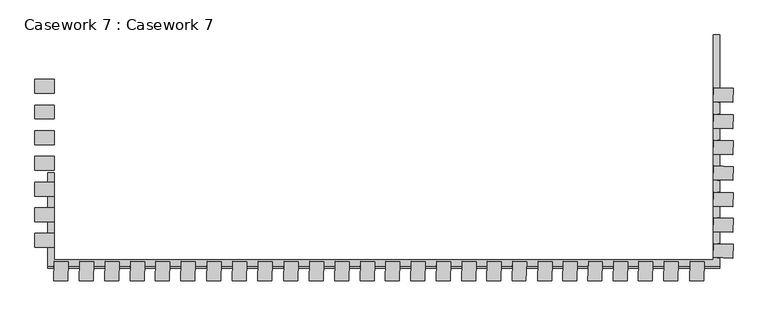
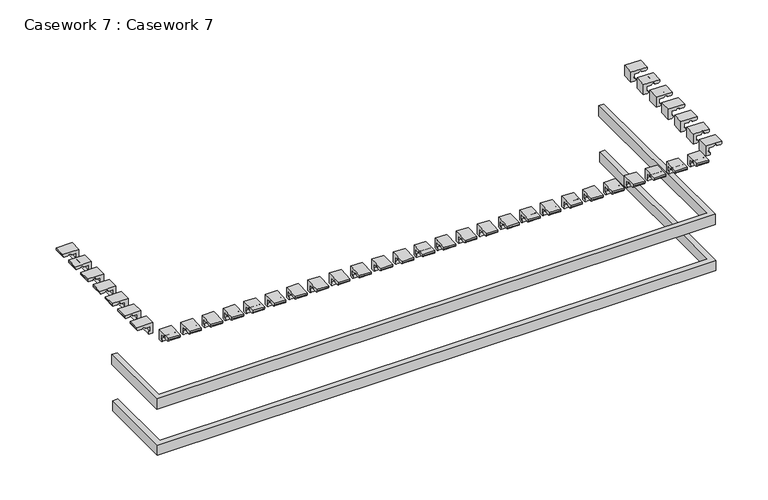
"""IFC4 building model written with IfcOpenShell, lengths in millimetres: furniture geometry, Casework 7 : Casework 7."""

from ifc_helpers import new_model, si_unit, point, frame, frame_2d, origin, place, context, project, spatial, polyline, circle_curve, trimmed, segment, composite_curve, outline, extrude, source, transform, mapped, element, save


def casework_7_casework_7_7bbf8f76(model_context):
    return source(origin(), model_context, "Body", "SweptSolid", [
        extrude(outline(composite_curve([segment(polyline([(0.0, 0.0), (15.0, 0.0)]), True, "CONTINUOUS"), segment(trimmed(circle_curve(frame_2d((15.0, -15.0)), 15.0), [point((15.0, 0.0))], [point((30.0, -15.0))], False, "CARTESIAN"), True, "CONTINUOUS"), segment(polyline([(30.0, -15.0), (30.0, -47.4999999)]), True, "CONTINUOUS"), segment(trimmed(circle_curve(frame_2d((30.0, -62.4999999)), 15.0), [point((30.0, -47.4999999))], [point((30.0, -77.5))], True, "CARTESIAN"), True, "CONTINUOUS"), segment(polyline([(30.0, -77.5), (30.0, -120.0), (70.0, -120.0)]), True, "CONTINUOUS"), segment(trimmed(circle_curve(frame_2d((85.0, -120.0)), 15.0), [point((70.0, -120.0))], [point((100.0, -120.0))], False, "CARTESIAN"), True, "CONTINUOUS"), segment(polyline([(100.0, -120.0), (100.0, -150.0), (0.0, -150.0), (0.0, 0.0)]), True, "CONTINUOUS")], self_intersect=False)), frame((3179.6256879, -13036.8692678, 4349.8564029), z_axis=(-0.9996210812387005, 0.02752624099239521, 0.0), x_axis=(0.0, 0.0, -1.0)), (0.0, 0.0, 1.0), 108.7993469),
        extrude(outline(composite_curve([segment(polyline([(0.0, 0.0), (15.0, 0.0)]), True, "CONTINUOUS"), segment(trimmed(circle_curve(frame_2d((15.0, -15.0)), 15.0), [point((15.0, 0.0))], [point((30.0, -15.0))], False, "CARTESIAN"), True, "CONTINUOUS"), segment(polyline([(30.0, -15.0), (30.0, -47.4999999)]), True, "CONTINUOUS"), segment(trimmed(circle_curve(frame_2d((30.0, -62.4999999)), 15.0), [point((30.0, -47.4999999))], [point((30.0, -77.5))], True, "CARTESIAN"), True, "CONTINUOUS"), segment(polyline([(30.0, -77.5), (30.0, -120.0), (70.0, -120.0)]), True, "CONTINUOUS"), segment(trimmed(circle_curve(frame_2d((85.0, -120.0)), 15.0), [point((70.0, -120.0))], [point((100.0, -120.0))], False, "CARTESIAN"), True, "CONTINUOUS"), segment(polyline([(100.0, -120.0), (100.0, -150.0), (0.0, -150.0), (0.0, 0.0)]), True, "CONTINUOUS")], self_intersect=False)), frame((2979.6256879, -13036.8692678, 4349.8564029), z_axis=(-0.9996210812387005, 0.02752624099239521, 0.0), x_axis=(0.0, 0.0, -1.0)), (0.0, 0.0, 1.0), 108.7993469),
        extrude(outline(composite_curve([segment(polyline([(0.0, 0.0), (15.0, 0.0)]), True, "CONTINUOUS"), segment(trimmed(circle_curve(frame_2d((15.0, -15.0)), 15.0), [point((15.0, 0.0))], [point((30.0, -15.0))], False, "CARTESIAN"), True, "CONTINUOUS"), segment(polyline([(30.0, -15.0), (30.0, -47.4999999)]), True, "CONTINUOUS"), segment(trimmed(circle_curve(frame_2d((30.0, -62.4999999)), 15.0), [point((30.0, -47.4999999))], [point((30.0, -77.5))], True, "CARTESIAN"), True, "CONTINUOUS"), segment(polyline([(30.0, -77.5), (30.0, -120.0), (70.0, -120.0)]), True, "CONTINUOUS"), segment(trimmed(circle_curve(frame_2d((85.0, -120.0)), 15.0), [point((70.0, -120.0))], [point((100.0, -120.0))], False, "CARTESIAN"), True, "CONTINUOUS"), segment(polyline([(100.0, -120.0), (100.0, -150.0), (0.0, -150.0), (0.0, 0.0)]), True, "CONTINUOUS")], self_intersect=False)), frame((2779.6256879, -13036.8692678, 4349.8564029), z_axis=(-0.9996210812387005, 0.02752624099239521, 0.0), x_axis=(0.0, 0.0, -1.0)), (0.0, 0.0, 1.0), 108.7993469),
        extrude(outline(composite_curve([segment(polyline([(0.0, 0.0), (15.0, 0.0)]), True, "CONTINUOUS"), segment(trimmed(circle_curve(frame_2d((15.0, -15.0)), 15.0), [point((15.0, 0.0))], [point((30.0, -15.0))], False, "CARTESIAN"), True, "CONTINUOUS"), segment(polyline([(30.0, -15.0), (30.0, -47.4999999)]), True, "CONTINUOUS"), segment(trimmed(circle_curve(frame_2d((30.0, -62.4999999)), 15.0), [point((30.0, -47.4999999))], [point((30.0, -77.5))], True, "CARTESIAN"), True, "CONTINUOUS"), segment(polyline([(30.0, -77.5), (30.0, -120.0), (70.0, -120.0)]), True, "CONTINUOUS"), segment(trimmed(circle_curve(frame_2d((85.0, -120.0)), 15.0), [point((70.0, -120.0))], [point((100.0, -120.0))], False, "CARTESIAN"), True, "CONTINUOUS"), segment(polyline([(100.0, -120.0), (100.0, -150.0), (0.0, -150.0), (0.0, 0.0)]), True, "CONTINUOUS")], self_intersect=False)), frame((2583.754624, -13036.8692678, 4349.8564029), z_axis=(-0.9996210812387005, 0.02752624099239521, 0.0), x_axis=(0.0, 0.0, -1.0)), (0.0, 0.0, 1.0), 108.7993469),
        extrude(outline(composite_curve([segment(polyline([(0.0, 0.0), (15.0, 0.0)]), True, "CONTINUOUS"), segment(trimmed(circle_curve(frame_2d((15.0, -15.0)), 15.0), [point((15.0, 0.0))], [point((30.0, -15.0))], False, "CARTESIAN"), True, "CONTINUOUS"), segment(polyline([(30.0, -15.0), (30.0, -47.4999999)]), True, "CONTINUOUS"), segment(trimmed(circle_curve(frame_2d((30.0, -62.4999999)), 15.0), [point((30.0, -47.4999999))], [point((30.0, -77.5))], True, "CARTESIAN"), True, "CONTINUOUS"), segment(polyline([(30.0, -77.5), (30.0, -120.0), (70.0, -120.0)]), True, "CONTINUOUS"), segment(trimmed(circle_curve(frame_2d((85.0, -120.0)), 15.0), [point((70.0, -120.0))], [point((100.0, -120.0))], False, "CARTESIAN"), True, "CONTINUOUS"), segment(polyline([(100.0, -120.0), (100.0, -150.0), (0.0, -150.0), (0.0, 0.0)]), True, "CONTINUOUS")], self_intersect=False)), frame((2387.8835602, -13036.8692678, 4349.8564029), z_axis=(-0.9996210812387005, 0.02752624099239521, 0.0), x_axis=(0.0, 0.0, -1.0)), (0.0, 0.0, 1.0), 108.7993469),
        extrude(outline(composite_curve([segment(polyline([(0.0, 0.0), (15.0, 0.0)]), True, "CONTINUOUS"), segment(trimmed(circle_curve(frame_2d((15.0, -15.0)), 15.0), [point((15.0, 0.0))], [point((30.0, -15.0))], False, "CARTESIAN"), True, "CONTINUOUS"), segment(polyline([(30.0, -15.0), (30.0, -47.4999999)]), True, "CONTINUOUS"), segment(trimmed(circle_curve(frame_2d((30.0, -62.4999999)), 15.0), [point((30.0, -47.4999999))], [point((30.0, -77.5))], True, "CARTESIAN"), True, "CONTINUOUS"), segment(polyline([(30.0, -77.5), (30.0, -120.0), (70.0, -120.0)]), True, "CONTINUOUS"), segment(trimmed(circle_curve(frame_2d((85.0, -120.0)), 15.0), [point((70.0, -120.0))], [point((100.0, -120.0))], False, "CARTESIAN"), True, "CONTINUOUS"), segment(polyline([(100.0, -120.0), (100.0, -150.0), (0.0, -150.0), (0.0, 0.0)]), True, "CONTINUOUS")], self_intersect=False)), frame((2192.0124963, -13036.8692678, 4349.8564029), z_axis=(-0.9996210812387005, 0.02752624099239521, 0.0), x_axis=(0.0, 0.0, -1.0)), (0.0, 0.0, 1.0), 108.7993469),
        extrude(outline(composite_curve([segment(polyline([(0.0, 0.0), (15.0, 0.0)]), True, "CONTINUOUS"), segment(trimmed(circle_curve(frame_2d((15.0, -15.0)), 15.0), [point((15.0, 0.0))], [point((30.0, -15.0))], False, "CARTESIAN"), True, "CONTINUOUS"), segment(polyline([(30.0, -15.0), (30.0, -47.4999999)]), True, "CONTINUOUS"), segment(trimmed(circle_curve(frame_2d((30.0, -62.4999999)), 15.0), [point((30.0, -47.4999999))], [point((30.0, -77.5))], True, "CARTESIAN"), True, "CONTINUOUS"), segment(polyline([(30.0, -77.5), (30.0, -120.0), (70.0, -120.0)]), True, "CONTINUOUS"), segment(trimmed(circle_curve(frame_2d((85.0, -120.0)), 15.0), [point((70.0, -120.0))], [point((100.0, -120.0))], False, "CARTESIAN"), True, "CONTINUOUS"), segment(polyline([(100.0, -120.0), (100.0, -150.0), (0.0, -150.0), (0.0, 0.0)]), True, "CONTINUOUS")], self_intersect=False)), frame((1996.1414325, -13036.8692678, 4349.8564029), z_axis=(-0.9996210812387005, 0.02752624099239521, 0.0), x_axis=(0.0, 0.0, -1.0)), (0.0, 0.0, 1.0), 108.7993469),
        extrude(outline(composite_curve([segment(polyline([(0.0, 0.0), (15.0, 0.0)]), True, "CONTINUOUS"), segment(trimmed(circle_curve(frame_2d((15.0, -15.0)), 15.0), [point((15.0, 0.0))], [point((30.0, -15.0))], False, "CARTESIAN"), True, "CONTINUOUS"), segment(polyline([(30.0, -15.0), (30.0, -47.4999999)]), True, "CONTINUOUS"), segment(trimmed(circle_curve(frame_2d((30.0, -62.4999999)), 15.0), [point((30.0, -47.4999999))], [point((30.0, -77.5))], True, "CARTESIAN"), True, "CONTINUOUS"), segment(polyline([(30.0, -77.5), (30.0, -120.0), (70.0, -120.0)]), True, "CONTINUOUS"), segment(trimmed(circle_curve(frame_2d((85.0, -120.0)), 15.0), [point((70.0, -120.0))], [point((100.0, -120.0))], False, "CARTESIAN"), True, "CONTINUOUS"), segment(polyline([(100.0, -120.0), (100.0, -150.0), (0.0, -150.0), (0.0, 0.0)]), True, "CONTINUOUS")], self_intersect=False)), frame((1796.1414325, -13036.8692678, 4349.8564029), z_axis=(-0.9996210812387005, 0.02752624099239521, 0.0), x_axis=(0.0, 0.0, -1.0)), (0.0, 0.0, 1.0), 108.7993469),
        extrude(outline(composite_curve([segment(polyline([(0.0, 0.0), (15.0, 0.0)]), True, "CONTINUOUS"), segment(trimmed(circle_curve(frame_2d((15.0, -15.0)), 15.0), [point((15.0, 0.0))], [point((30.0, -15.0))], False, "CARTESIAN"), True, "CONTINUOUS"), segment(polyline([(30.0, -15.0), (30.0, -47.4999999)]), True, "CONTINUOUS"), segment(trimmed(circle_curve(frame_2d((30.0, -62.4999999)), 15.0), [point((30.0, -47.4999999))], [point((30.0, -77.5))], True, "CARTESIAN"), True, "CONTINUOUS"), segment(polyline([(30.0, -77.5), (30.0, -120.0), (70.0, -120.0)]), True, "CONTINUOUS"), segment(trimmed(circle_curve(frame_2d((85.0, -120.0)), 15.0), [point((70.0, -120.0))], [point((100.0, -120.0))], False, "CARTESIAN"), True, "CONTINUOUS"), segment(polyline([(100.0, -120.0), (100.0, -150.0), (0.0, -150.0), (0.0, 0.0)]), True, "CONTINUOUS")], self_intersect=False)), frame((1600.2703686, -13036.8692678, 4349.8564029), z_axis=(-0.9996210812387005, 0.02752624099239521, 0.0), x_axis=(0.0, 0.0, -1.0)), (0.0, 0.0, 1.0), 108.7993469),
        extrude(outline(composite_curve([segment(polyline([(0.0, 0.0), (15.0, 0.0)]), True, "CONTINUOUS"), segment(trimmed(circle_curve(frame_2d((15.0, -15.0)), 15.0), [point((15.0, 0.0))], [point((30.0, -15.0))], False, "CARTESIAN"), True, "CONTINUOUS"), segment(polyline([(30.0, -15.0), (30.0, -47.4999999)]), True, "CONTINUOUS"), segment(trimmed(circle_curve(frame_2d((30.0, -62.4999999)), 15.0), [point((30.0, -47.4999999))], [point((30.0, -77.5))], True, "CARTESIAN"), True, "CONTINUOUS"), segment(polyline([(30.0, -77.5), (30.0, -120.0), (70.0, -120.0)]), True, "CONTINUOUS"), segment(trimmed(circle_curve(frame_2d((85.0, -120.0)), 15.0), [point((70.0, -120.0))], [point((100.0, -120.0))], False, "CARTESIAN"), True, "CONTINUOUS"), segment(polyline([(100.0, -120.0), (100.0, -150.0), (0.0, -150.0), (0.0, 0.0)]), True, "CONTINUOUS")], self_intersect=False)), frame((1404.3993048, -13036.8692678, 4349.8564029), z_axis=(-0.9996210812387005, 0.02752624099239521, 0.0), x_axis=(0.0, 0.0, -1.0)), (0.0, 0.0, 1.0), 108.7993469),
        extrude(outline(composite_curve([segment(polyline([(0.0, 0.0), (15.0, 0.0)]), True, "CONTINUOUS"), segment(trimmed(circle_curve(frame_2d((15.0, -15.0)), 15.0), [point((15.0, 0.0))], [point((30.0, -15.0))], False, "CARTESIAN"), True, "CONTINUOUS"), segment(polyline([(30.0, -15.0), (30.0, -47.4999999)]), True, "CONTINUOUS"), segment(trimmed(circle_curve(frame_2d((30.0, -62.4999999)), 15.0), [point((30.0, -47.4999999))], [point((30.0, -77.5))], True, "CARTESIAN"), True, "CONTINUOUS"), segment(polyline([(30.0, -77.5), (30.0, -120.0), (70.0, -120.0)]), True, "CONTINUOUS"), segment(trimmed(circle_curve(frame_2d((85.0, -120.0)), 15.0), [point((70.0, -120.0))], [point((100.0, -120.0))], False, "CARTESIAN"), True, "CONTINUOUS"), segment(polyline([(100.0, -120.0), (100.0, -150.0), (0.0, -150.0), (0.0, 0.0)]), True, "CONTINUOUS")], self_intersect=False)), frame((1204.3993048, -13036.8692678, 4349.8564029), z_axis=(-0.9996210812387005, 0.02752624099239521, 0.0), x_axis=(0.0, 0.0, -1.0)), (0.0, 0.0, 1.0), 108.7993469),
        extrude(outline(composite_curve([segment(polyline([(0.0, 0.0), (15.0, 0.0)]), True, "CONTINUOUS"), segment(trimmed(circle_curve(frame_2d((15.0, -15.0)), 15.0), [point((15.0, 0.0))], [point((30.0, -15.0))], False, "CARTESIAN"), True, "CONTINUOUS"), segment(polyline([(30.0, -15.0), (30.0, -47.4999999)]), True, "CONTINUOUS"), segment(trimmed(circle_curve(frame_2d((30.0, -62.4999999)), 15.0), [point((30.0, -47.4999999))], [point((30.0, -77.5))], True, "CARTESIAN"), True, "CONTINUOUS"), segment(polyline([(30.0, -77.5), (30.0, -120.0), (70.0, -120.0)]), True, "CONTINUOUS"), segment(trimmed(circle_curve(frame_2d((85.0, -120.0)), 15.0), [point((70.0, -120.0))], [point((100.0, -120.0))], False, "CARTESIAN"), True, "CONTINUOUS"), segment(polyline([(100.0, -120.0), (100.0, -150.0), (0.0, -150.0), (0.0, 0.0)]), True, "CONTINUOUS")], self_intersect=False)), frame((1008.5282409, -13036.8692678, 4349.8564029), z_axis=(-0.9996210812387005, 0.02752624099239521, 0.0), x_axis=(0.0, 0.0, -1.0)), (0.0, 0.0, 1.0), 108.7993469),
        extrude(outline(composite_curve([segment(polyline([(0.0, 0.0), (15.0, 0.0)]), True, "CONTINUOUS"), segment(trimmed(circle_curve(frame_2d((15.0, -15.0)), 15.0), [point((15.0, 0.0))], [point((30.0, -15.0))], False, "CARTESIAN"), True, "CONTINUOUS"), segment(polyline([(30.0, -15.0), (30.0, -47.4999999)]), True, "CONTINUOUS"), segment(trimmed(circle_curve(frame_2d((30.0, -62.4999999)), 15.0), [point((30.0, -47.4999999))], [point((30.0, -77.5))], True, "CARTESIAN"), True, "CONTINUOUS"), segment(polyline([(30.0, -77.5), (30.0, -120.0), (70.0, -120.0)]), True, "CONTINUOUS"), segment(trimmed(circle_curve(frame_2d((85.0, -120.0)), 15.0), [point((70.0, -120.0))], [point((100.0, -120.0))], False, "CARTESIAN"), True, "CONTINUOUS"), segment(polyline([(100.0, -120.0), (100.0, -150.0), (0.0, -150.0), (0.0, 0.0)]), True, "CONTINUOUS")], self_intersect=False)), frame((808.5282409, -13036.8692678, 4349.8564029), z_axis=(-0.9996210812387005, 0.02752624099239521, 0.0), x_axis=(0.0, 0.0, -1.0)), (0.0, 0.0, 1.0), 108.7993469),
        extrude(outline(composite_curve([segment(polyline([(0.0, 0.0), (15.0, 0.0)]), True, "CONTINUOUS"), segment(trimmed(circle_curve(frame_2d((15.0, -15.0)), 15.0), [point((15.0, 0.0))], [point((30.0, -15.0))], False, "CARTESIAN"), True, "CONTINUOUS"), segment(polyline([(30.0, -15.0), (30.0, -47.4999999)]), True, "CONTINUOUS"), segment(trimmed(circle_curve(frame_2d((30.0, -62.4999999)), 15.0), [point((30.0, -47.4999999))], [point((30.0, -77.5))], True, "CARTESIAN"), True, "CONTINUOUS"), segment(polyline([(30.0, -77.5), (30.0, -120.0), (70.0, -120.0)]), True, "CONTINUOUS"), segment(trimmed(circle_curve(frame_2d((85.0, -120.0)), 15.0), [point((70.0, -120.0))], [point((100.0, -120.0))], False, "CARTESIAN"), True, "CONTINUOUS"), segment(polyline([(100.0, -120.0), (100.0, -150.0), (0.0, -150.0), (0.0, 0.0)]), True, "CONTINUOUS")], self_intersect=False)), frame((612.6571771, -13036.8692678, 4349.8564029), z_axis=(-0.9996210812387005, 0.02752624099239521, 0.0), x_axis=(0.0, 0.0, -1.0)), (0.0, 0.0, 1.0), 108.7993469),
        extrude(outline(composite_curve([segment(polyline([(0.0, 0.0), (15.0, 0.0)]), True, "CONTINUOUS"), segment(trimmed(circle_curve(frame_2d((15.0, -15.0)), 15.0), [point((15.0, 0.0))], [point((30.0, -15.0))], False, "CARTESIAN"), True, "CONTINUOUS"), segment(polyline([(30.0, -15.0), (30.0, -47.4999999)]), True, "CONTINUOUS"), segment(trimmed(circle_curve(frame_2d((30.0, -62.4999999)), 15.0), [point((30.0, -47.4999999))], [point((30.0, -77.5))], True, "CARTESIAN"), True, "CONTINUOUS"), segment(polyline([(30.0, -77.5), (30.0, -120.0), (70.0, -120.0)]), True, "CONTINUOUS"), segment(trimmed(circle_curve(frame_2d((85.0, -120.0)), 15.0), [point((70.0, -120.0))], [point((100.0, -120.0))], False, "CARTESIAN"), True, "CONTINUOUS"), segment(polyline([(100.0, -120.0), (100.0, -150.0), (0.0, -150.0), (0.0, 0.0)]), True, "CONTINUOUS")], self_intersect=False)), frame((416.7861132, -13036.8692678, 4349.8564029), z_axis=(-0.9996210812387005, 0.02752624099239521, 0.0), x_axis=(0.0, 0.0, -1.0)), (0.0, 0.0, 1.0), 108.7993469),
        extrude(outline(composite_curve([segment(polyline([(0.0, 0.0), (15.0, 0.0)]), True, "CONTINUOUS"), segment(trimmed(circle_curve(frame_2d((15.0, -15.0)), 15.0), [point((15.0, 0.0))], [point((30.0, -15.0))], False, "CARTESIAN"), True, "CONTINUOUS"), segment(polyline([(30.0, -15.0), (30.0, -47.4999999)]), True, "CONTINUOUS"), segment(trimmed(circle_curve(frame_2d((30.0, -62.4999999)), 15.0), [point((30.0, -47.4999999))], [point((30.0, -77.5))], True, "CARTESIAN"), True, "CONTINUOUS"), segment(polyline([(30.0, -77.5), (30.0, -120.0), (70.0, -120.0)]), True, "CONTINUOUS"), segment(trimmed(circle_curve(frame_2d((85.0, -120.0)), 15.0), [point((70.0, -120.0))], [point((100.0, -120.0))], False, "CARTESIAN"), True, "CONTINUOUS"), segment(polyline([(100.0, -120.0), (100.0, -150.0), (0.0, -150.0), (0.0, 0.0)]), True, "CONTINUOUS")], self_intersect=False)), frame((216.7861132, -13036.8692678, 4349.8564029), z_axis=(-0.9996210812387005, 0.02752624099239521, 0.0), x_axis=(0.0, 0.0, -1.0)), (0.0, 0.0, 1.0), 108.7993469),
        extrude(outline(composite_curve([segment(polyline([(0.0, 0.0), (15.0, 0.0)]), True, "CONTINUOUS"), segment(trimmed(circle_curve(frame_2d((15.0, -15.0)), 15.0), [point((15.0, 0.0))], [point((30.0, -15.0))], False, "CARTESIAN"), True, "CONTINUOUS"), segment(polyline([(30.0, -15.0), (30.0, -47.4999999)]), True, "CONTINUOUS"), segment(trimmed(circle_curve(frame_2d((30.0, -62.4999999)), 15.0), [point((30.0, -47.4999999))], [point((30.0, -77.5))], True, "CARTESIAN"), True, "CONTINUOUS"), segment(polyline([(30.0, -77.5), (30.0, -120.0), (70.0, -120.0)]), True, "CONTINUOUS"), segment(trimmed(circle_curve(frame_2d((85.0, -120.0)), 15.0), [point((70.0, -120.0))], [point((100.0, -120.0))], False, "CARTESIAN"), True, "CONTINUOUS"), segment(polyline([(100.0, -120.0), (100.0, -150.0), (0.0, -150.0), (0.0, 0.0)]), True, "CONTINUOUS")], self_intersect=False)), frame((16.7861132, -13036.8692678, 4349.8564029), z_axis=(-0.9996210812387005, 0.02752624099239521, 0.0), x_axis=(0.0, 0.0, -1.0)), (0.0, 0.0, 1.0), 108.7993469),
        extrude(outline(composite_curve([segment(polyline([(0.0, 0.0), (15.0, 0.0)]), True, "CONTINUOUS"), segment(trimmed(circle_curve(frame_2d((15.0, -15.0)), 15.0), [point((15.0, 0.0))], [point((30.0, -15.0))], False, "CARTESIAN"), True, "CONTINUOUS"), segment(polyline([(30.0, -15.0), (30.0, -47.4999999)]), True, "CONTINUOUS"), segment(trimmed(circle_curve(frame_2d((30.0, -62.4999999)), 15.0), [point((30.0, -47.4999999))], [point((30.0, -77.5))], True, "CARTESIAN"), True, "CONTINUOUS"), segment(polyline([(30.0, -77.5), (30.0, -120.0), (70.0, -120.0)]), True, "CONTINUOUS"), segment(trimmed(circle_curve(frame_2d((85.0, -120.0)), 15.0), [point((70.0, -120.0))], [point((100.0, -120.0))], False, "CARTESIAN"), True, "CONTINUOUS"), segment(polyline([(100.0, -120.0), (100.0, -150.0), (0.0, -150.0), (0.0, 0.0)]), True, "CONTINUOUS")], self_intersect=False)), frame((-183.2138868, -13036.8692678, 4349.8564029), z_axis=(-0.9996210812387005, 0.02752624099239521, 0.0), x_axis=(0.0, 0.0, -1.0)), (0.0, 0.0, 1.0), 108.7993469),
        extrude(outline(composite_curve([segment(polyline([(0.0, 0.0), (15.0, 0.0)]), True, "CONTINUOUS"), segment(trimmed(circle_curve(frame_2d((15.0, -15.0)), 15.0), [point((15.0, 0.0))], [point((30.0, -15.0))], False, "CARTESIAN"), True, "CONTINUOUS"), segment(polyline([(30.0, -15.0), (30.0, -47.4999999)]), True, "CONTINUOUS"), segment(trimmed(circle_curve(frame_2d((30.0, -62.4999999)), 15.0), [point((30.0, -47.4999999))], [point((30.0, -77.5))], True, "CARTESIAN"), True, "CONTINUOUS"), segment(polyline([(30.0, -77.5), (30.0, -120.0), (70.0, -120.0)]), True, "CONTINUOUS"), segment(trimmed(circle_curve(frame_2d((85.0, -120.0)), 15.0), [point((70.0, -120.0))], [point((100.0, -120.0))], False, "CARTESIAN"), True, "CONTINUOUS"), segment(polyline([(100.0, -120.0), (100.0, -150.0), (0.0, -150.0), (0.0, 0.0)]), True, "CONTINUOUS")], self_intersect=False)), frame((-383.2138868, -13036.8692678, 4349.8564029), z_axis=(-0.9996210812387005, 0.02752624099239521, 0.0), x_axis=(0.0, 0.0, -1.0)), (0.0, 0.0, 1.0), 108.7993469),
        extrude(outline(composite_curve([segment(polyline([(0.0, 0.0), (15.0, 0.0)]), True, "CONTINUOUS"), segment(trimmed(circle_curve(frame_2d((15.0, -15.0)), 15.0), [point((15.0, 0.0))], [point((30.0, -15.0))], False, "CARTESIAN"), True, "CONTINUOUS"), segment(polyline([(30.0, -15.0), (30.0, -47.4999999)]), True, "CONTINUOUS"), segment(trimmed(circle_curve(frame_2d((30.0, -62.4999999)), 15.0), [point((30.0, -47.4999999))], [point((30.0, -77.5))], True, "CARTESIAN"), True, "CONTINUOUS"), segment(polyline([(30.0, -77.5), (30.0, -120.0), (70.0, -120.0)]), True, "CONTINUOUS"), segment(trimmed(circle_curve(frame_2d((85.0, -120.0)), 15.0), [point((70.0, -120.0))], [point((100.0, -120.0))], False, "CARTESIAN"), True, "CONTINUOUS"), segment(polyline([(100.0, -120.0), (100.0, -150.0), (0.0, -150.0), (0.0, 0.0)]), True, "CONTINUOUS")], self_intersect=False)), frame((-583.2138868, -13036.8692678, 4349.8564029), z_axis=(-0.9996210812387005, 0.02752624099239521, 0.0), x_axis=(0.0, 0.0, -1.0)), (0.0, 0.0, 1.0), 108.7993469),
        extrude(outline(composite_curve([segment(polyline([(0.0, 0.0), (15.0, 0.0)]), True, "CONTINUOUS"), segment(trimmed(circle_curve(frame_2d((15.0, -15.0)), 15.0), [point((15.0, 0.0))], [point((30.0, -15.0))], False, "CARTESIAN"), True, "CONTINUOUS"), segment(polyline([(30.0, -15.0), (30.0, -47.4999999)]), True, "CONTINUOUS"), segment(trimmed(circle_curve(frame_2d((30.0, -62.4999999)), 15.0), [point((30.0, -47.4999999))], [point((30.0, -77.5))], True, "CARTESIAN"), True, "CONTINUOUS"), segment(polyline([(30.0, -77.5), (30.0, -120.0), (70.0, -120.0)]), True, "CONTINUOUS"), segment(trimmed(circle_curve(frame_2d((85.0, -120.0)), 15.0), [point((70.0, -120.0))], [point((100.0, -120.0))], False, "CARTESIAN"), True, "CONTINUOUS"), segment(polyline([(100.0, -120.0), (100.0, -150.0), (0.0, -150.0), (0.0, 0.0)]), True, "CONTINUOUS")], self_intersect=False)), frame((-783.2138868, -13036.8692678, 4349.8564029), z_axis=(-0.9996210812387005, 0.02752624099239521, 0.0), x_axis=(0.0, 0.0, -1.0)), (0.0, 0.0, 1.0), 108.7993469),
        extrude(outline(composite_curve([segment(polyline([(0.0, 0.0), (15.0, 0.0)]), True, "CONTINUOUS"), segment(trimmed(circle_curve(frame_2d((15.0, -15.0)), 15.0), [point((15.0, 0.0))], [point((30.0, -15.0))], False, "CARTESIAN"), True, "CONTINUOUS"), segment(polyline([(30.0, -15.0), (30.0, -47.4999999)]), True, "CONTINUOUS"), segment(trimmed(circle_curve(frame_2d((30.0, -62.4999999)), 15.0), [point((30.0, -47.4999999))], [point((30.0, -77.5))], True, "CARTESIAN"), True, "CONTINUOUS"), segment(polyline([(30.0, -77.5), (30.0, -120.0), (70.0, -120.0)]), True, "CONTINUOUS"), segment(trimmed(circle_curve(frame_2d((85.0, -120.0)), 15.0), [point((70.0, -120.0))], [point((100.0, -120.0))], False, "CARTESIAN"), True, "CONTINUOUS"), segment(polyline([(100.0, -120.0), (100.0, -150.0), (0.0, -150.0), (0.0, 0.0)]), True, "CONTINUOUS")], self_intersect=False)), frame((-983.2138868, -13036.8692678, 4349.8564029), z_axis=(-0.9996210812387005, 0.02752624099239521, 0.0), x_axis=(0.0, 0.0, -1.0)), (0.0, 0.0, 1.0), 108.7993469),
        extrude(outline(composite_curve([segment(polyline([(0.0, 0.0), (15.0, 0.0)]), True, "CONTINUOUS"), segment(trimmed(circle_curve(frame_2d((15.0, -15.0)), 15.0), [point((15.0, 0.0))], [point((30.0, -15.0))], False, "CARTESIAN"), True, "CONTINUOUS"), segment(polyline([(30.0, -15.0), (30.0, -47.4999999)]), True, "CONTINUOUS"), segment(trimmed(circle_curve(frame_2d((30.0, -62.4999999)), 15.0), [point((30.0, -47.4999999))], [point((30.0, -77.5))], True, "CARTESIAN"), True, "CONTINUOUS"), segment(polyline([(30.0, -77.5), (30.0, -120.0), (70.0, -120.0)]), True, "CONTINUOUS"), segment(trimmed(circle_curve(frame_2d((85.0, -120.0)), 15.0), [point((70.0, -120.0))], [point((100.0, -120.0))], False, "CARTESIAN"), True, "CONTINUOUS"), segment(polyline([(100.0, -120.0), (100.0, -150.0), (0.0, -150.0), (0.0, 0.0)]), True, "CONTINUOUS")], self_intersect=False)), frame((-1179.0849506, -13036.8692678, 4349.8564029), z_axis=(-0.9996210812387005, 0.02752624099239521, 0.0), x_axis=(0.0, 0.0, -1.0)), (0.0, 0.0, 1.0), 108.7993469),
        extrude(outline(composite_curve([segment(polyline([(0.0, 0.0), (15.0, 0.0)]), True, "CONTINUOUS"), segment(trimmed(circle_curve(frame_2d((15.0, -15.0)), 15.0), [point((15.0, 0.0))], [point((30.0, -15.0))], False, "CARTESIAN"), True, "CONTINUOUS"), segment(polyline([(30.0, -15.0), (30.0, -47.4999999)]), True, "CONTINUOUS"), segment(trimmed(circle_curve(frame_2d((30.0, -62.4999999)), 15.0), [point((30.0, -47.4999999))], [point((30.0, -77.5))], True, "CARTESIAN"), True, "CONTINUOUS"), segment(polyline([(30.0, -77.5), (30.0, -120.0), (70.0, -120.0)]), True, "CONTINUOUS"), segment(trimmed(circle_curve(frame_2d((85.0, -120.0)), 15.0), [point((70.0, -120.0))], [point((100.0, -120.0))], False, "CARTESIAN"), True, "CONTINUOUS"), segment(polyline([(100.0, -120.0), (100.0, -150.0), (0.0, -150.0), (0.0, 0.0)]), True, "CONTINUOUS")], self_intersect=False)), frame((-1374.9560145, -13036.8692678, 4349.8564029), z_axis=(-0.9996210812387005, 0.02752624099239521, 0.0), x_axis=(0.0, 0.0, -1.0)), (0.0, 0.0, 1.0), 108.7993469),
        extrude(outline(composite_curve([segment(polyline([(0.0, 0.0), (15.0, 0.0)]), True, "CONTINUOUS"), segment(trimmed(circle_curve(frame_2d((15.0, -15.0)), 15.0), [point((15.0, 0.0))], [point((30.0, -15.0))], False, "CARTESIAN"), True, "CONTINUOUS"), segment(polyline([(30.0, -15.0), (30.0, -47.4999999)]), True, "CONTINUOUS"), segment(trimmed(circle_curve(frame_2d((30.0, -62.4999999)), 15.0), [point((30.0, -47.4999999))], [point((30.0, -77.5))], True, "CARTESIAN"), True, "CONTINUOUS"), segment(polyline([(30.0, -77.5), (30.0, -120.0), (70.0, -120.0)]), True, "CONTINUOUS"), segment(trimmed(circle_curve(frame_2d((85.0, -120.0)), 15.0), [point((70.0, -120.0))], [point((100.0, -120.0))], False, "CARTESIAN"), True, "CONTINUOUS"), segment(polyline([(100.0, -120.0), (100.0, -150.0), (0.0, -150.0), (0.0, 0.0)]), True, "CONTINUOUS")], self_intersect=False)), frame((-1574.9560145, -13036.8692678, 4349.8564029), z_axis=(-0.9996210812387005, 0.02752624099239521, 0.0), x_axis=(0.0, 0.0, -1.0)), (0.0, 0.0, 1.0), 108.7993469),
        extrude(outline(composite_curve([segment(polyline([(0.0, 0.0), (15.0, 0.0)]), True, "CONTINUOUS"), segment(trimmed(circle_curve(frame_2d((15.0, -15.0)), 15.0), [point((15.0, 0.0))], [point((30.0, -15.0))], False, "CARTESIAN"), True, "CONTINUOUS"), segment(polyline([(30.0, -15.0), (30.0, -47.4999999)]), True, "CONTINUOUS"), segment(trimmed(circle_curve(frame_2d((30.0, -62.4999999)), 15.0), [point((30.0, -47.4999999))], [point((30.0, -77.5))], True, "CARTESIAN"), True, "CONTINUOUS"), segment(polyline([(30.0, -77.5), (30.0, -120.0), (70.0, -120.0)]), True, "CONTINUOUS"), segment(trimmed(circle_curve(frame_2d((85.0, -120.0)), 15.0), [point((70.0, -120.0))], [point((100.0, -120.0))], False, "CARTESIAN"), True, "CONTINUOUS"), segment(polyline([(100.0, -120.0), (100.0, -150.0), (0.0, -150.0), (0.0, 0.0)]), True, "CONTINUOUS")], self_intersect=False)), frame((-1774.9560145, -13036.8692678, 4349.8564029), z_axis=(-0.9996210812387005, 0.02752624099239521, 0.0), x_axis=(0.0, 0.0, -1.0)), (0.0, 0.0, 1.0), 108.7993469),
        extrude(outline(composite_curve([segment(polyline([(0.0, 0.0), (0.0, -150.0), (-100.0, -150.0), (-100.0, -120.0)]), True, "CONTINUOUS"), segment(trimmed(circle_curve(frame_2d((-85.0, -120.0)), 15.0), [point((-100.0, -120.0))], [point((-70.0, -120.0))], False, "CARTESIAN"), True, "CONTINUOUS"), segment(polyline([(-70.0, -120.0), (-30.0, -120.0), (-30.0, -77.5)]), True, "CONTINUOUS"), segment(trimmed(circle_curve(frame_2d((-30.0, -62.5)), 15.0), [point((-30.0, -77.5))], [point((-30.0, -47.4999999))], True, "CARTESIAN"), True, "CONTINUOUS"), segment(polyline([(-30.0, -47.4999999), (-30.0, -15.0)]), True, "CONTINUOUS"), segment(trimmed(circle_curve(frame_2d((-15.0, -15.0)), 15.0), [point((-30.0, -15.0))], [point((-15.0, 0.0))], False, "CARTESIAN"), True, "CONTINUOUS"), segment(polyline([(-15.0, 0.0), (0.0, 0.0)]), True, "CONTINUOUS")], self_intersect=False)), frame((3406.5339649, -11646.2525329, 4349.8564029), z_axis=(0.027526240992393435, 0.9996210812387005, 0.0), x_axis=(0.0, 0.0, 1.0)), (0.0, 0.0, 1.0), 108.7993469),
        extrude(outline(composite_curve([segment(polyline([(0.0, 0.0), (0.0, -150.0), (-100.0, -150.0), (-100.0, -120.0)]), True, "CONTINUOUS"), segment(trimmed(circle_curve(frame_2d((-85.0, -120.0)), 15.0), [point((-100.0, -120.0))], [point((-70.0, -120.0))], False, "CARTESIAN"), True, "CONTINUOUS"), segment(polyline([(-70.0, -120.0), (-30.0, -120.0), (-30.0, -77.5)]), True, "CONTINUOUS"), segment(trimmed(circle_curve(frame_2d((-30.0, -62.5)), 15.0), [point((-30.0, -77.5))], [point((-30.0, -47.4999999))], True, "CARTESIAN"), True, "CONTINUOUS"), segment(polyline([(-30.0, -47.4999999), (-30.0, -15.0)]), True, "CONTINUOUS"), segment(trimmed(circle_curve(frame_2d((-15.0, -15.0)), 15.0), [point((-30.0, -15.0))], [point((-15.0, 0.0))], False, "CARTESIAN"), True, "CONTINUOUS"), segment(polyline([(-15.0, 0.0), (0.0, 0.0)]), True, "CONTINUOUS")], self_intersect=False)), frame((3406.5339649, -11850.381469, 4349.8564029), z_axis=(0.027526240992393435, 0.9996210812387005, 0.0), x_axis=(0.0, 0.0, 1.0)), (0.0, 0.0, 1.0), 108.7993469),
        extrude(outline(composite_curve([segment(polyline([(0.0, 0.0), (0.0, -150.0), (-100.0, -150.0), (-100.0, -120.0)]), True, "CONTINUOUS"), segment(trimmed(circle_curve(frame_2d((-85.0, -120.0)), 15.0), [point((-100.0, -120.0))], [point((-70.0, -120.0))], False, "CARTESIAN"), True, "CONTINUOUS"), segment(polyline([(-70.0, -120.0), (-30.0, -120.0), (-30.0, -77.5)]), True, "CONTINUOUS"), segment(trimmed(circle_curve(frame_2d((-30.0, -62.5)), 15.0), [point((-30.0, -77.5))], [point((-30.0, -47.4999999))], True, "CARTESIAN"), True, "CONTINUOUS"), segment(polyline([(-30.0, -47.4999999), (-30.0, -15.0)]), True, "CONTINUOUS"), segment(trimmed(circle_curve(frame_2d((-15.0, -15.0)), 15.0), [point((-30.0, -15.0))], [point((-15.0, 0.0))], False, "CARTESIAN"), True, "CONTINUOUS"), segment(polyline([(-15.0, 0.0), (0.0, 0.0)]), True, "CONTINUOUS")], self_intersect=False)), frame((3406.5339649, -12054.5104052, 4349.8564029), z_axis=(0.027526240992393435, 0.9996210812387005, 0.0), x_axis=(0.0, 0.0, 1.0)), (0.0, 0.0, 1.0), 108.7993469),
        extrude(outline(composite_curve([segment(polyline([(0.0, 0.0), (0.0, -150.0), (-100.0, -150.0), (-100.0, -120.0)]), True, "CONTINUOUS"), segment(trimmed(circle_curve(frame_2d((-85.0, -120.0)), 15.0), [point((-100.0, -120.0))], [point((-70.0, -120.0))], False, "CARTESIAN"), True, "CONTINUOUS"), segment(polyline([(-70.0, -120.0), (-30.0, -120.0), (-30.0, -77.5)]), True, "CONTINUOUS"), segment(trimmed(circle_curve(frame_2d((-30.0, -62.5)), 15.0), [point((-30.0, -77.5))], [point((-30.0, -47.4999999))], True, "CARTESIAN"), True, "CONTINUOUS"), segment(polyline([(-30.0, -47.4999999), (-30.0, -15.0)]), True, "CONTINUOUS"), segment(trimmed(circle_curve(frame_2d((-15.0, -15.0)), 15.0), [point((-30.0, -15.0))], [point((-15.0, 0.0))], False, "CARTESIAN"), True, "CONTINUOUS"), segment(polyline([(-15.0, 0.0), (0.0, 0.0)]), True, "CONTINUOUS")], self_intersect=False)), frame((3406.5339649, -12254.5104052, 4349.8564029), z_axis=(0.027526240992393435, 0.9996210812387005, 0.0), x_axis=(0.0, 0.0, 1.0)), (0.0, 0.0, 1.0), 108.7993469),
        extrude(outline(composite_curve([segment(polyline([(0.0, 0.0), (0.0, -150.0), (-100.0, -150.0), (-100.0, -120.0)]), True, "CONTINUOUS"), segment(trimmed(circle_curve(frame_2d((-85.0, -120.0)), 15.0), [point((-100.0, -120.0))], [point((-70.0, -120.0))], False, "CARTESIAN"), True, "CONTINUOUS"), segment(polyline([(-70.0, -120.0), (-30.0, -120.0), (-30.0, -77.5)]), True, "CONTINUOUS"), segment(trimmed(circle_curve(frame_2d((-30.0, -62.5)), 15.0), [point((-30.0, -77.5))], [point((-30.0, -47.4999999))], True, "CARTESIAN"), True, "CONTINUOUS"), segment(polyline([(-30.0, -47.4999999), (-30.0, -15.0)]), True, "CONTINUOUS"), segment(trimmed(circle_curve(frame_2d((-15.0, -15.0)), 15.0), [point((-30.0, -15.0))], [point((-15.0, 0.0))], False, "CARTESIAN"), True, "CONTINUOUS"), segment(polyline([(-15.0, 0.0), (0.0, 0.0)]), True, "CONTINUOUS")], self_intersect=False)), frame((3406.5339649, -12458.6393413, 4349.8564029), z_axis=(0.027526240992393435, 0.9996210812387005, 0.0), x_axis=(0.0, 0.0, 1.0)), (0.0, 0.0, 1.0), 108.7993469),
        extrude(outline(composite_curve([segment(polyline([(0.0, 0.0), (0.0, -150.0), (-100.0, -150.0), (-100.0, -120.0)]), True, "CONTINUOUS"), segment(trimmed(circle_curve(frame_2d((-85.0, -120.0)), 15.0), [point((-100.0, -120.0))], [point((-70.0, -120.0))], False, "CARTESIAN"), True, "CONTINUOUS"), segment(polyline([(-70.0, -120.0), (-30.0, -120.0), (-30.0, -77.5)]), True, "CONTINUOUS"), segment(trimmed(circle_curve(frame_2d((-30.0, -62.5)), 15.0), [point((-30.0, -77.5))], [point((-30.0, -47.4999999))], True, "CARTESIAN"), True, "CONTINUOUS"), segment(polyline([(-30.0, -47.4999999), (-30.0, -15.0)]), True, "CONTINUOUS"), segment(trimmed(circle_curve(frame_2d((-15.0, -15.0)), 15.0), [point((-30.0, -15.0))], [point((-15.0, 0.0))], False, "CARTESIAN"), True, "CONTINUOUS"), segment(polyline([(-15.0, 0.0), (0.0, 0.0)]), True, "CONTINUOUS")], self_intersect=False)), frame((3406.5339649, -12658.6393413, 4349.8564029), z_axis=(0.027526240992393435, 0.9996210812387005, 0.0), x_axis=(0.0, 0.0, 1.0)), (0.0, 0.0, 1.0), 108.7993469),
        extrude(outline(composite_curve([segment(polyline([(0.0, 0.0), (0.0, -150.0), (-100.0, -150.0), (-100.0, -120.0)]), True, "CONTINUOUS"), segment(trimmed(circle_curve(frame_2d((-85.0, -120.0)), 15.0), [point((-100.0, -120.0))], [point((-70.0, -120.0))], False, "CARTESIAN"), True, "CONTINUOUS"), segment(polyline([(-70.0, -120.0), (-30.0, -120.0), (-30.0, -77.5)]), True, "CONTINUOUS"), segment(trimmed(circle_curve(frame_2d((-30.0, -62.5)), 15.0), [point((-30.0, -77.5))], [point((-30.0, -47.4999999))], True, "CARTESIAN"), True, "CONTINUOUS"), segment(polyline([(-30.0, -47.4999999), (-30.0, -15.0)]), True, "CONTINUOUS"), segment(trimmed(circle_curve(frame_2d((-15.0, -15.0)), 15.0), [point((-30.0, -15.0))], [point((-15.0, 0.0))], False, "CARTESIAN"), True, "CONTINUOUS"), segment(polyline([(-15.0, 0.0), (0.0, 0.0)]), True, "CONTINUOUS")], self_intersect=False)), frame((3406.5339649, -12858.6393413, 4349.8564029), z_axis=(0.027526240992393435, 0.9996210812387005, 0.0), x_axis=(0.0, 0.0, 1.0)), (0.0, 0.0, 1.0), 108.7993469),
        extrude(outline(composite_curve([segment(polyline([(4349.8564029, -2029.2953966), (4334.8564029, -2029.2953966)]), True, "CONTINUOUS"), segment(trimmed(circle_curve(frame_2d((4334.8564029, -2014.2953966)), 15.0), [point((4334.8564029, -2029.2953966))], [point((4319.8564029, -2014.2953966))], False, "CARTESIAN"), True, "CONTINUOUS"), segment(polyline([(4319.8564029, -2014.2953966), (4319.8564029, -1981.7953966)]), True, "CONTINUOUS"), segment(trimmed(circle_curve(frame_2d((4319.8564029, -1966.7953966)), 15.0), [point((4319.8564029, -1981.7953966))], [point((4319.8564029, -1951.7953966))], True, "CARTESIAN"), True, "CONTINUOUS"), segment(polyline([(4319.8564029, -1951.7953966), (4319.8564029, -1909.2953966), (4279.8564029, -1909.2953966)]), True, "CONTINUOUS"), segment(trimmed(circle_curve(frame_2d((4264.8564029, -1909.2953966)), 15.0), [point((4279.8564029, -1909.2953966))], [point((4249.8564029, -1909.2953966))], False, "CARTESIAN"), True, "CONTINUOUS"), segment(polyline([(4249.8564029, -1909.2953966), (4249.8564029, -1879.2953966), (4349.8564029, -1879.2953966), (4349.8564029, -2029.2953966)]), True, "CONTINUOUS")], self_intersect=False)), frame((0.0, -12775.4922632, 0.0), z_axis=(0.0, 1.0, 0.0), x_axis=(0.0, 0.0, 1.0)), (0.0, 0.0, 1.0), 108.7993469),
        extrude(outline(composite_curve([segment(polyline([(4349.8564029, -2029.2953966), (4334.8564029, -2029.2953966)]), True, "CONTINUOUS"), segment(trimmed(circle_curve(frame_2d((4334.8564029, -2014.2953966)), 15.0), [point((4334.8564029, -2029.2953966))], [point((4319.8564029, -2014.2953966))], False, "CARTESIAN"), True, "CONTINUOUS"), segment(polyline([(4319.8564029, -2014.2953966), (4319.8564029, -1981.7953966)]), True, "CONTINUOUS"), segment(trimmed(circle_curve(frame_2d((4319.8564029, -1966.7953966)), 15.0), [point((4319.8564029, -1981.7953966))], [point((4319.8564029, -1951.7953966))], True, "CARTESIAN"), True, "CONTINUOUS"), segment(polyline([(4319.8564029, -1951.7953966), (4319.8564029, -1909.2953966), (4279.8564029, -1909.2953966)]), True, "CONTINUOUS"), segment(trimmed(circle_curve(frame_2d((4264.8564029, -1909.2953966)), 15.0), [point((4279.8564029, -1909.2953966))], [point((4249.8564029, -1909.2953966))], False, "CARTESIAN"), True, "CONTINUOUS"), segment(polyline([(4249.8564029, -1909.2953966), (4249.8564029, -1879.2953966), (4349.8564029, -1879.2953966), (4349.8564029, -2029.2953966)]), True, "CONTINUOUS")], self_intersect=False)), frame((0.0, -12575.4922632, 0.0), z_axis=(0.0, 1.0, 0.0), x_axis=(0.0, 0.0, 1.0)), (0.0, 0.0, 1.0), 108.7993469),
        extrude(outline(composite_curve([segment(polyline([(4349.8564029, -2029.2953966), (4334.8564029, -2029.2953966)]), True, "CONTINUOUS"), segment(trimmed(circle_curve(frame_2d((4334.8564029, -2014.2953966)), 15.0), [point((4334.8564029, -2029.2953966))], [point((4319.8564029, -2014.2953966))], False, "CARTESIAN"), True, "CONTINUOUS"), segment(polyline([(4319.8564029, -2014.2953966), (4319.8564029, -1981.7953966)]), True, "CONTINUOUS"), segment(trimmed(circle_curve(frame_2d((4319.8564029, -1966.7953966)), 15.0), [point((4319.8564029, -1981.7953966))], [point((4319.8564029, -1951.7953966))], True, "CARTESIAN"), True, "CONTINUOUS"), segment(polyline([(4319.8564029, -1951.7953966), (4319.8564029, -1909.2953966), (4279.8564029, -1909.2953966)]), True, "CONTINUOUS"), segment(trimmed(circle_curve(frame_2d((4264.8564029, -1909.2953966)), 15.0), [point((4279.8564029, -1909.2953966))], [point((4249.8564029, -1909.2953966))], False, "CARTESIAN"), True, "CONTINUOUS"), segment(polyline([(4249.8564029, -1909.2953966), (4249.8564029, -1879.2953966), (4349.8564029, -1879.2953966), (4349.8564029, -2029.2953966)]), True, "CONTINUOUS")], self_intersect=False)), frame((0.0, -12375.4922632, 0.0), z_axis=(0.0, 1.0, 0.0), x_axis=(0.0, 0.0, 1.0)), (0.0, 0.0, 1.0), 108.7993469),
        extrude(outline(composite_curve([segment(polyline([(4349.8564029, -2029.2953966), (4334.8564029, -2029.2953966)]), True, "CONTINUOUS"), segment(trimmed(circle_curve(frame_2d((4334.8564029, -2014.2953966)), 15.0), [point((4334.8564029, -2029.2953966))], [point((4319.8564029, -2014.2953966))], False, "CARTESIAN"), True, "CONTINUOUS"), segment(polyline([(4319.8564029, -2014.2953966), (4319.8564029, -1981.7953966)]), True, "CONTINUOUS"), segment(trimmed(circle_curve(frame_2d((4319.8564029, -1966.7953966)), 15.0), [point((4319.8564029, -1981.7953966))], [point((4319.8564029, -1951.7953966))], True, "CARTESIAN"), True, "CONTINUOUS"), segment(polyline([(4319.8564029, -1951.7953966), (4319.8564029, -1909.2953966), (4279.8564029, -1909.2953966)]), True, "CONTINUOUS"), segment(trimmed(circle_curve(frame_2d((4264.8564029, -1909.2953966)), 15.0), [point((4279.8564029, -1909.2953966))], [point((4249.8564029, -1909.2953966))], False, "CARTESIAN"), True, "CONTINUOUS"), segment(polyline([(4249.8564029, -1909.2953966), (4249.8564029, -1879.2953966), (4349.8564029, -1879.2953966), (4349.8564029, -2029.2953966)]), True, "CONTINUOUS")], self_intersect=False)), frame((0.0, -12175.4922632, 0.0), z_axis=(0.0, 1.0, 0.0), x_axis=(0.0, 0.0, 1.0)), (0.0, 0.0, 1.0), 108.7993469),
        extrude(outline(composite_curve([segment(polyline([(4349.8564029, -2029.2953966), (4334.8564029, -2029.2953966)]), True, "CONTINUOUS"), segment(trimmed(circle_curve(frame_2d((4334.8564029, -2014.2953966)), 15.0), [point((4334.8564029, -2029.2953966))], [point((4319.8564029, -2014.2953966))], False, "CARTESIAN"), True, "CONTINUOUS"), segment(polyline([(4319.8564029, -2014.2953966), (4319.8564029, -1981.7953966)]), True, "CONTINUOUS"), segment(trimmed(circle_curve(frame_2d((4319.8564029, -1966.7953966)), 15.0), [point((4319.8564029, -1981.7953966))], [point((4319.8564029, -1951.7953966))], True, "CARTESIAN"), True, "CONTINUOUS"), segment(polyline([(4319.8564029, -1951.7953966), (4319.8564029, -1909.2953966), (4279.8564029, -1909.2953966)]), True, "CONTINUOUS"), segment(trimmed(circle_curve(frame_2d((4264.8564029, -1909.2953966)), 15.0), [point((4279.8564029, -1909.2953966))], [point((4249.8564029, -1909.2953966))], False, "CARTESIAN"), True, "CONTINUOUS"), segment(polyline([(4249.8564029, -1909.2953966), (4249.8564029, -1879.2953966), (4349.8564029, -1879.2953966), (4349.8564029, -2029.2953966)]), True, "CONTINUOUS")], self_intersect=False)), frame((0.0, -11975.4922632, 0.0), z_axis=(0.0, 1.0, 0.0), x_axis=(0.0, 0.0, 1.0)), (0.0, 0.0, 1.0), 108.7993469),
        extrude(outline(composite_curve([segment(polyline([(4349.8564029, -2029.2953966), (4334.8564029, -2029.2953966)]), True, "CONTINUOUS"), segment(trimmed(circle_curve(frame_2d((4334.8564029, -2014.2953966)), 15.0), [point((4334.8564029, -2029.2953966))], [point((4319.8564029, -2014.2953966))], False, "CARTESIAN"), True, "CONTINUOUS"), segment(polyline([(4319.8564029, -2014.2953966), (4319.8564029, -1981.7953966)]), True, "CONTINUOUS"), segment(trimmed(circle_curve(frame_2d((4319.8564029, -1966.7953966)), 15.0), [point((4319.8564029, -1981.7953966))], [point((4319.8564029, -1951.7953966))], True, "CARTESIAN"), True, "CONTINUOUS"), segment(polyline([(4319.8564029, -1951.7953966), (4319.8564029, -1909.2953966), (4279.8564029, -1909.2953966)]), True, "CONTINUOUS"), segment(trimmed(circle_curve(frame_2d((4264.8564029, -1909.2953966)), 15.0), [point((4279.8564029, -1909.2953966))], [point((4249.8564029, -1909.2953966))], False, "CARTESIAN"), True, "CONTINUOUS"), segment(polyline([(4249.8564029, -1909.2953966), (4249.8564029, -1879.2953966), (4349.8564029, -1879.2953966), (4349.8564029, -2029.2953966)]), True, "CONTINUOUS")], self_intersect=False)), frame((0.0, -11775.4922632, 0.0), z_axis=(0.0, 1.0, 0.0), x_axis=(0.0, 0.0, 1.0)), (0.0, 0.0, 1.0), 108.7993469),
        extrude(outline(composite_curve([segment(polyline([(4349.8564029, -2029.2953966), (4334.8564029, -2029.2953966)]), True, "CONTINUOUS"), segment(trimmed(circle_curve(frame_2d((4334.8564029, -2014.2953966)), 15.0), [point((4334.8564029, -2029.2953966))], [point((4319.8564029, -2014.2953966))], False, "CARTESIAN"), True, "CONTINUOUS"), segment(polyline([(4319.8564029, -2014.2953966), (4319.8564029, -1981.7953966)]), True, "CONTINUOUS"), segment(trimmed(circle_curve(frame_2d((4319.8564029, -1966.7953966)), 15.0), [point((4319.8564029, -1981.7953966))], [point((4319.8564029, -1951.7953966))], True, "CARTESIAN"), True, "CONTINUOUS"), segment(polyline([(4319.8564029, -1951.7953966), (4319.8564029, -1909.2953966), (4279.8564029, -1909.2953966)]), True, "CONTINUOUS"), segment(trimmed(circle_curve(frame_2d((4264.8564029, -1909.2953966)), 15.0), [point((4279.8564029, -1909.2953966))], [point((4249.8564029, -1909.2953966))], False, "CARTESIAN"), True, "CONTINUOUS"), segment(polyline([(4249.8564029, -1909.2953966), (4249.8564029, -1879.2953966), (4349.8564029, -1879.2953966), (4349.8564029, -2029.2953966)]), True, "CONTINUOUS")], self_intersect=False)), frame((0.0, -11575.4922632, 0.0), z_axis=(0.0, 1.0, 0.0), x_axis=(0.0, 0.0, 1.0)), (0.0, 0.0, 1.0), 108.7993469),
        extrude(outline(polyline([(-1929.2953966, -12195.5500949), (-1879.2953966, -12195.5500949), (-1879.2953966, -12873.0500949), (3255.7046034, -12873.0500949), (3255.7046034, -11120.5500949), (3305.7046034, -11120.5500949), (3305.7046034, -12923.0500949), (-1929.2953966, -12923.0500949), (-1929.2953966, -12195.5500949)])), frame((0.0, 0.0, 3599.3782897), z_axis=(0.0, 0.0, 1.0), x_axis=(1.0, 0.0, 0.0)), (0.0, 0.0, 1.0), 100.0),
        extrude(outline(polyline([(-1929.2953966, -12209.1929163), (-1879.2953966, -12209.1929163), (-1879.2953966, -12886.6929163), (3255.7046034, -12886.6929163), (3255.7046034, -11134.1929163), (3305.7046034, -11134.1929163), (3305.7046034, -12936.6929163), (-1929.2953966, -12936.6929163), (-1929.2953966, -12209.1929163)])), frame((0.0, 0.0, 3150.0), z_axis=(0.0, 0.0, 1.0), x_axis=(1.0, 0.0, 0.0)), (0.0, 0.0, 1.0), 100.0),
    ])


if __name__ == "__main__":
    model = new_model("IFC4")
    model_context = context("Model", 3, world=origin())
    ifc_project = project(units=[si_unit("LENGTHUNIT", "METRE", prefix="MILLI")], contexts=[model_context])
    site = spatial("IfcSite", under=ifc_project)
    building = spatial("IfcBuilding", under=site)
    placement = place(None, origin())
    casework_7_casework_7_shape = casework_7_casework_7_7bbf8f76(model_context)
    element("IfcFurniture", 1, ObjectType="Casework 7 : Casework 7", at=placement, inside=building, context=model_context, shape_type="MappedRepresentation", body=[
        mapped(casework_7_casework_7_shape, transform((0.0, 0.0, 0.0), x_axis=(1.0, 0.0, 0.0), y_axis=(0.0, 1.0, 0.0), z_axis=(0.0, 0.0, 1.0))),
    ])
    save(model, "model.ifc")
